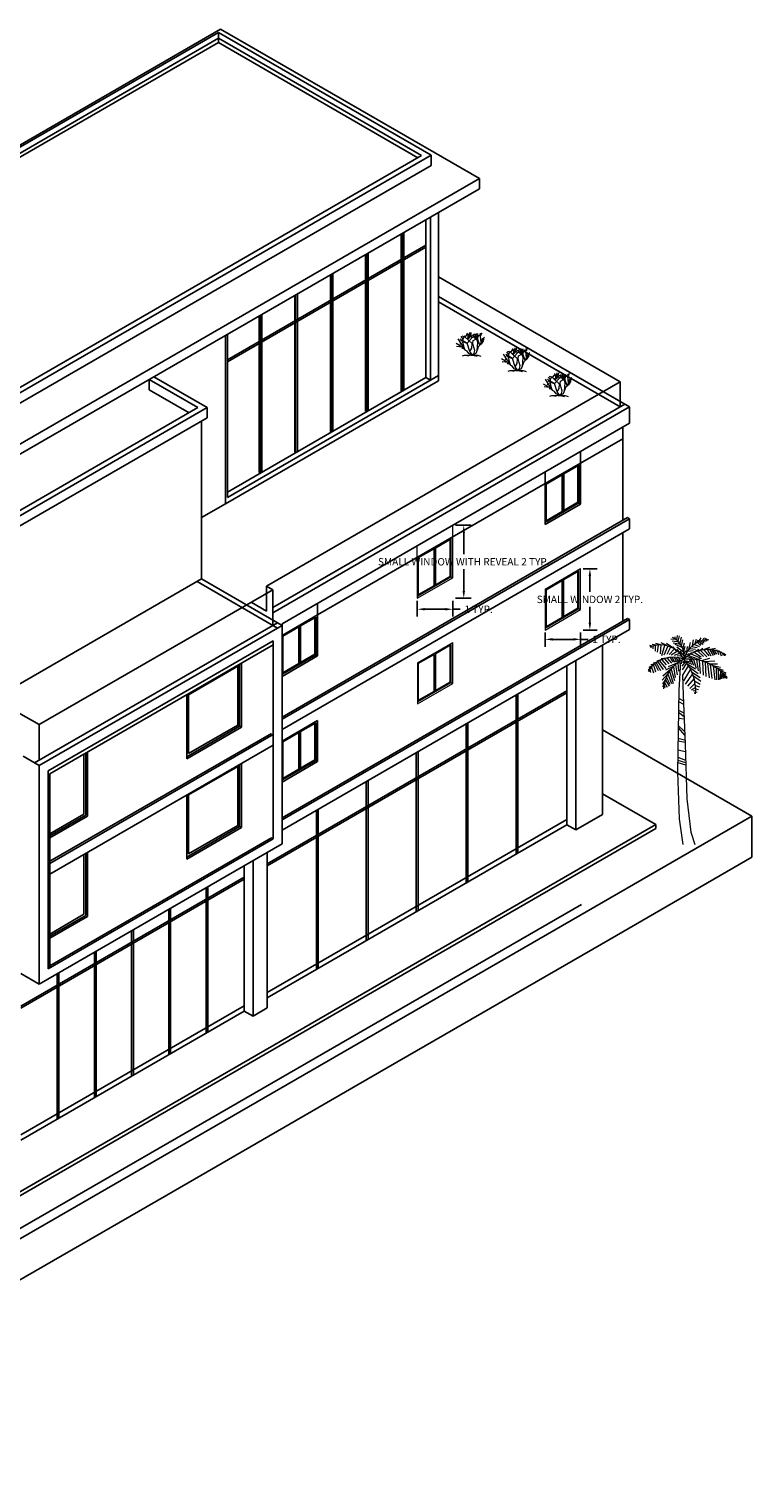
# Model space of a CAD drawing. Units: metres. Extents: x 20738 to 41533, y 14777 to 29586.
# Tile 2 of 2: x 20763 to 20780, y 14778 to 14814. Entities that reach past the tile are written whole.
import ezdxf

# ---------------------------------------------------------------- set-up
doc = ezdxf.new("R2010")
doc.units = ezdxf.units.M
for name, color, linetype, lineweight in [('A-ANNO-DIMS', 2, 'Continuous', 18), ('A-ANNO-NPLT', 8, 'Continuous', 13), ('A-ELEV', 7, 'Continuous', 25), ('A-GLAZ', 4, 'Continuous', 18), ('L-PLNT', 92, 'Continuous', 13)]:
    doc.layers.add(name, color=color, linetype=linetype, lineweight=lineweight)
doc.styles.get("Standard").update_dxf_attribs({"font": 'arial.ttf'})
doc.dimstyles.get("Standard").update_dxf_attribs({"dimtxt": 0.18, "dimasz": 0.18, "dimexe": 0.18, "dimexo": 0.0625, "dimgap": 0.09, "dimtad": 0, "dimtih": 1, "dimtoh": 1, "dimdec": 4, "dimzin": 0, "dimdsep": 46, "dimtxsty": 'Standard', "dimcen": 0.09, "dimadec": 0, "dimazin": 0, "dimtfac": 1, "dimtdec": 4, "dimtofl": 0, "dimtmove": 0, "dimatfit": 3, "dimfxl": 1, "dimtolj": 1, "dimtzin": 0, "dimarcsym": 0})

# ---------------------------------------------------------------- blocks, each defined once
blk = doc.blocks.new('*U2')
for p, q in [((-18.24, 11.04), (-21.755, 16.655)), ((-12.96, 12.48), (-19.68, 16.32)), ((-13.92, 12.48), (-19.2, 14.88)), ((-16.8, 16.32), (-18.72, 18.72)), ((-14.88, 18.24), (-17.76, 19.2)), ((-16.8, 16.32), (-15.36, 19.68)), ((-16.8, 12.48), (-16.8, 16.32)), ((-14.88, 18.24), (-12.96, 20.64)), ((-8.16, 12), (-14.88, 18.24)), ((-13.325, 16.724), (-11.433, 18.289)), ((-12.96, 12.48), (-8.16, 17.76)), ((-12.471, 19.775), (-12.898, 22.044)), ((-11.677, 19.071), (-12.471, 19.775)), ((-11.28, 19.619), (-12.104, 21.184)), ((-12.043, 15.628), (-11.921, 18.836)), ((-11.982, 16.802), (-10.579, 18.054)), ((-11.921, 18.836), (-10.64, 20.401)), ((-11.433, 18.289), (-10.457, 22.749)), ((-10.579, 18.054), (-9.846, 19.697)), ((-8.16, 17.76), (-10.56, 21.6)), ((-9.48, 19.775), (-8.992, 22.592)), ((-7.2, 19.68), (-8.64, 20.16)), ((-8.16, 17.76), (-5.28, 19.2)), ((-7.68, 12.48), (-7.2, 14.88)), ((-7.2, 19.68), (-6.24, 21.12)), ((-4.8, 16.32), (-7.2, 19.68)), ((-7.2, 14.88), (-3.84, 16.8)), ((-5.086, 17.741), (-5.513, 21.34)), ((-5.28, 19.2), (-3.84, 21.6)), ((-3.377, 15.315), (-5.086, 17.819)), ((-2.88, 12.96), (-4.32, 19.68)), ((-3.84, 16.8), (-0.96, 20.64)), ((-3.377, 18.602), (-2.888, 21.575)), ((-2.766, 16.802), (-3.377, 18.602)), ((-2.88, 15.84), (-2.4, 20.16)), ((-0.96, 10.56), (-2.88, 15.84)), ((-0.508, 21.888), (-0.081, 20.558)), ((-0.203, 19.149), (0.102, 21.34)), ((0.346, 13.203), (-0.203, 19.149)), ((-0.142, 19.384), (0.59, 20.401)), ((-0.02, 20.01), (0.896, 21.105)), ((0.041, 20.714), (1.384, 22.044)), ((0.102, 21.34), (0.835, 21.888)), ((0.346, 13.203), (1.323, 16.254)), ((0.96, 12), (1.44, 15.36)), ((0.96, 12), (2.88, 14.88)), ((1.323, 16.254), (3.642, 18.289)), ((1.44, 15.36), (2.88, 17.28)), ((1.92, 13.44), (2.4, 15.36)), ((2.4, 15.36), (3.36, 16.32)), ((-17.76, 8.64), (-23.663, 11.961)), ((-17.76, 8.64), (-23.128, 9.222)), ((-18.24, 11.04), (-20.16, 11.52)), ((-15.84, 8.16), (-18.24, 11.04)), ((-16.32, 7.2), (-18.24, 7.2)), ((-16.8, 12.48), (-17.76, 12.96)), ((-14.88, 5.76), (-17.76, 8.64)), ((-15.84, 0.48), (-17.76, 0)), ((-15.84, 8.16), (-16.8, 12.48)), ((-14.88, 5.76), (-15.84, 8.16)), ((-13.44, 0.48), (-15.84, 0.48)), ((-12.96, 4.8), (-14.88, 5.76)), ((-12.96, 12.48), (-13.92, 12.48)), ((-9.6, 0.96), (-13.44, 0.48)), ((-10.56, 4.32), (-12.96, 12.48)), ((-11.52, 2.4), (-12.96, 4.8)), ((-9.6, 0.96), (-12.96, 0)), ((-8.64, 0.96), (-11.52, 2.4)), ((-10.56, 4.32), (-8.64, 7.68)), ((-8.64, 1.92), (-10.56, 4.32)), ((-9.6, 0.96), (-7.68, 0.96)), ((-8.64, 7.68), (-8.16, 12)), ((-8.64, 0.96), (-4.32, 2.88)), ((-8.64, 0.96), (-6.24, 2.88)), ((-8.64, 0.96), (-8.64, 1.92)), ((-8.64, 0.96), (-2.88, 0.96)), ((-6.72, 8.64), (-7.68, 12.48)), ((-7.68, 0.96), (-6.24, 0.48)), ((-5.76, 5.28), (-6.72, 8.64)), ((-6.24, 2.88), (-5.76, 5.28)), ((-6.24, 0.48), (-3.36, 0)), ((-4.32, 2.88), (-1.92, 9.6)), ((-3.36, 5.28), (-2.88, 12.96)), ((-2.88, 0.96), (0, 0)), ((-1.92, 9.6), (0.96, 12)), ((-0.48, 10.8), (0.346, 13.203))]:
    blk.add_line(p, q)
blk = doc.blocks.new('*U4')
for p, q in [((-6.727, 197.202), (-11.366, 197.45)), ((-3.441, 194.477), (-10.013, 195.716)), ((-7.5, 199.68), (-7.5, 197.946)), ((-5.567, 196.707), (-4.987, 201.167)), ((-4.407, 195.716), (-3.247, 200.672)), ((-2.474, 193.733), (-1.315, 199.433)), ((-1.121, 190.759), (0.232, 196.955)), ((9.317, 191.255), (10.283, 196.955)), ((11.829, 192.99), (13.182, 197.45)), ((13.956, 194.229), (14.729, 196.955)), ((15.116, 194.477), (17.822, 198.689)), ((18.015, 195.716), (20.914, 198.689)), ((19.368, 196.459), (19.948, 193.733)), ((20.914, 196.459), (21.301, 194.972)), ((21.301, 196.459), (22.847, 198.441)), ((22.074, 196.707), (23.427, 195.716)), ((23.234, 196.707), (23.62, 197.698)), ((-29.729, 190.759), (-31.469, 191.255)), ((-30.309, 190.512), (-30.695, 189.025)), ((-25.283, 191.751), (-29.342, 192.246)), ((-28.763, 190.759), (-28.763, 188.281)), ((-26.443, 191.503), (-26.636, 186.051)), ((-20.064, 191.751), (-25.863, 193.238)), ((-23.737, 191.751), (-24.51, 185.06)), ((-21.031, 191.998), (-21.804, 183.325)), ((-15.232, 191.255), (-20.644, 193.981)), ((-17.551, 191.503), (-20.451, 181.343)), ((-14.265, 190.759), (-18.131, 182.086)), ((-9.433, 189.025), (-15.618, 193.238)), ((-11.753, 189.768), (-15.425, 182.83)), ((-8.08, 188.034), (-12.912, 182.83)), ((-4.987, 185.803), (-10.979, 182.086)), ((-1.894, 192.494), (-9.24, 193.733)), ((-6.147, 186.299), (-9.24, 190.264)), ((-3.247, 183.821), (-8.08, 181.838)), ((-0.541, 189.52), (-7.307, 192.494)), ((-5.76, 190.016), (0.618, 185.308)), ((-5.76, 188.034), (-1.508, 182.582)), ((-2.668, 185.803), (1.198, 181.343)), ((0.038, 188.281), (1.778, 193.981)), ((1.005, 185.803), (2.358, 190.759)), ((1.005, 182.582), (2.938, 186.547)), ((2.938, 182.582), (6.61, 183.821)), ((4.098, 185.06), (4.678, 190.512)), ((4.871, 186.051), (10.09, 186.547)), ((4.871, 181.591), (8.544, 184.812)), ((5.644, 181.838), (13.569, 178.865)), ((5.837, 187.786), (7.577, 194.229)), ((6.997, 188.529), (12.216, 187.786)), ((7.77, 183.325), (16.082, 179.856)), ((8.544, 190.512), (13.763, 189.52)), ((9.51, 184.317), (15.502, 188.034)), ((11.25, 192.494), (15.889, 190.512)), ((11.25, 184.812), (17.628, 180.352)), ((14.536, 193.981), (17.242, 191.255)), ((14.536, 185.803), (19.948, 180.847)), ((15.695, 186.299), (19.368, 188.777)), ((16.082, 194.972), (17.822, 192.494)), ((17.242, 186.547), (23.041, 180.599)), ((18.015, 195.468), (18.981, 192.494)), ((19.368, 187.29), (26.133, 189.768)), ((20.721, 187.042), (25.167, 181.343)), ((23.814, 187.29), (26.907, 181.343)), ((24.78, 187.538), (31.546, 188.777)), ((26.133, 187.29), (29.419, 181.838)), ((28.066, 187.29), (30.966, 182.582)), ((29.806, 186.795), (32.319, 183.078)), ((29.999, 186.795), (33.092, 187.29)), ((32.512, 186.299), (35.218, 186.299)), ((33.479, 186.051), (34.445, 182.83)), ((35.605, 185.556), (37.151, 185.308)), ((35.798, 185.308), (36.958, 181.591)), ((38.118, 184.317), (38.504, 181.838)), ((39.857, 182.83), (40.244, 181.591)), ((-32.628, 167.961), (-33.208, 167.961)), ((-32.628, 167.713), (-32.435, 165.979)), ((-28.956, 172.174), (-32.435, 170.192)), ((-31.082, 169.944), (-32.435, 169.2)), ((-31.662, 168.705), (-31.082, 165.483)), ((-27.409, 173.413), (-30.695, 172.67)), ((-29.922, 170.687), (-27.989, 165.235)), ((-25.09, 175.148), (-28.376, 174.404)), ((-27.989, 172.422), (-26.056, 166.227)), ((-26.829, 173.661), (-23.544, 167.218)), ((-25.476, 174.652), (-21.224, 167.466)), ((-21.031, 177.626), (-24.897, 176.387)), ((-24.317, 175.891), (-18.711, 168.457)), ((-22.191, 176.635), (-16.391, 169.448)), ((-15.618, 179.36), (-20.644, 178.617)), ((-20.064, 177.626), (-15.812, 172.67)), ((-12.139, 167.961), (-19.098, 162.014)), ((-17.358, 178.617), (-13.299, 173.661)), ((-8.466, 171.678), (-16.585, 167.713)), ((-15.038, 179.36), (-10.786, 174.404)), ((-4.214, 175.148), (-14.072, 170.935)), ((-12.332, 180.104), (-9.433, 175.643)), ((-10.979, 168.457), (-7.887, 157.801)), ((-10.206, 180.104), (-8.08, 175.891)), ((-8.853, 170.935), (-7.113, 160.527)), ((-1.701, 176.882), (-8.66, 175.396)), ((-8.273, 180.104), (-6.147, 176.635)), ((-6.92, 172.917), (-5.374, 163.253)), ((-6.34, 179.608), (-4.6, 177.13)), ((-1.315, 181.591), (-5.374, 181.095)), ((-4.6, 174.9), (-4.021, 166.722)), ((-4.021, 179.36), (-2.861, 177.378)), ((-2.668, 176.387), (-2.376, 170.594)), ((-0.348, 180.352), (-1.894, 180.104)), ((-0.928, 176.882), (-1.508, 173.909)), ((2.551, 175.891), (-0.928, 171.431)), ((3.711, 174.404), (-0.541, 167.961)), ((5.257, 171.926), (-0.155, 163.005)), ((1.585, 177.13), (0.038, 174.652)), ((7.384, 168.705), (0.812, 157.553)), ((1.585, 177.13), (6.61, 176.139)), ((2.938, 175.891), (8.737, 173.413)), ((4.098, 180.847), (8.35, 179.608)), ((4.291, 173.909), (12.216, 168.953)), ((6.224, 178.121), (8.157, 175.148)), ((6.417, 170.439), (14.729, 164.492)), ((7.384, 178.369), (10.476, 179.36)), ((8.157, 178.121), (10.476, 172.422)), ((10.476, 177.874), (12.796, 169.696)), ((11.829, 177.874), (18.015, 179.113)), ((13.182, 177.874), (14.729, 166.97)), ((15.889, 177.13), (16.855, 164.492)), ((18.015, 177.13), (26.133, 179.113)), ((18.981, 175.891), (19.561, 163.005)), ((20.914, 175.891), (30.966, 176.635)), ((21.688, 175.396), (22.074, 161.518)), ((23.814, 174.404), (25.554, 160.279)), ((25.554, 173.661), (33.285, 173.661)), ((26.52, 173.165), (28.066, 159.784)), ((28.839, 172.174), (36.378, 170.687)), ((29.226, 171.926), (30.966, 158.545)), ((30.966, 170.687), (38.891, 167.713)), ((32.126, 169.696), (32.512, 158.545)), ((34.058, 168.705), (34.445, 158.545)), ((35.412, 167.713), (41.404, 164.988)), ((-14.265, 164.244), (-19.678, 158.049)), ((-16.005, 160.031), (-19.484, 154.084)), ((-17.358, 155.819), (-14.845, 151.358)), ((-16.585, 158.545), (-13.106, 152.35)), ((-15.618, 160.775), (-12.332, 154.332)), ((-14.265, 163.749), (-10.786, 154.828)), ((-12.719, 166.722), (-9.046, 154.828)), ((9.317, 164.244), (2.358, 154.332)), ((10.863, 159.784), (4.484, 152.35)), ((11.829, 155.075), (6.804, 150.119)), ((8.544, 165.979), (16.662, 160.527)), ((10.09, 162.51), (17.435, 157.058)), ((11.443, 157.553), (16.855, 154.332)), ((36.378, 166.474), (35.605, 158.792)), ((37.731, 165.235), (36.958, 159.288)), ((37.924, 165.235), (41.404, 163.749)), ((38.504, 164.492), (38.504, 159.536)), ((39.664, 163.253), (42.37, 161.766)), ((39.857, 162.757), (39.857, 160.031)), ((40.824, 161.766), (41.21, 160.031)), ((41.21, 161.518), (42.757, 160.279)), ((-18.131, 153.589), (-19.484, 151.606)), ((-17.938, 152.597), (-16.972, 151.111)), ((-4.081, 140.645), (0.753, 138.261)), ((12.603, 151.111), (8.544, 148.385)), ((12.216, 148.137), (10.09, 147.393)), ((12.409, 145.659), (11.056, 145.659)), ((12.216, 153.093), (16.082, 151.606)), ((12.409, 146.898), (13.763, 146.402)), ((12.603, 149.872), (15.116, 149.128)), ((-4.081, 137.547), (0.753, 135.163)), ((-4.081, 129.205), (1.124, 126.821)), ((-4.081, 127.298), (1.31, 123.246)), ((-4.453, 112.283), (1.682, 105.133)), ((-4.267, 114.428), (1.682, 108.708)), ((-4.081, 121.578), (1.31, 120.863)), ((-4.639, 102.273), (1.868, 100.604)), ((-4.453, 99.651), (2.24, 98.459)), ((-4.825, 83.921), (2.612, 81.061)), ((-4.453, 91.071), (2.426, 89.641)), ((-4.639, 81.299), (2.797, 78.916)), ((-4.639, 78.916), (2.797, 76.771))]:
    blk.add_line(p, q)
for points in [[(-2.363, 170.553), (-3.88, 148.505), (-4.988, 69.634), (-3.325, 24.869), (0, 0)], [(-0.116, 162.848), (0.554, 143.532), (2.217, 96.635), (3.88, 44.054), (7.76, 12.079), (11.64, 0)]]:
    blk.add_lwpolyline(points)
for centre, radius, start, end in [((-18.427, 181.448), 19.715, 350.285, 64.11229), ((25.595, 171.567), 25.395, 91.40319, 163.882), ((-21.738, 166.094), 25.899, 27.67115, 112.5305), ((23.687, 155.341), 32.188, 56.19272, 134.3213), ((-9.259, 151.732), 28.386, 68.38311, 147.5322), ((14.394, 148.393), 32.752, 113.7592, 177.4133), ((5.828, 132.718), 45.639, 35.98777, 95.82273), ((-32.8, 147.923), 45.309, 356.1943, 41.37848)]:
    blk.add_arc(centre, radius, start, end)
blk = doc.blocks.new('WIN-SMALL')
for p, q in [((0, 1), (0.866, 1.5)), ((0.454, 1.235), (0.822, 1.448)), ((0.8, 0.54), (0.8, 1.435)), ((0.822, 0.525), (0.822, 1.448)), ((0.866, 0.5), (0.866, 1.5)), ((0.021, 0.985), (0.411, 1.21)), ((0.411, 0.315), (0.411, 1.21)), ((0.454, 0.34), (0.454, 1.235)), ((0, 1), (0, 0)), ((0.021, 0.985), (0.021, 0.062)), ((0, 0), (0.866, 0.5)), ((0.021, 0.062), (0.822, 0.525)), ((0.454, 0.34), (0.8, 0.54)), ((0.798, 0.538), (0.866, 0.5)), ((0.021, 0.09), (0.411, 0.315))]:
    blk.add_line(p, q)
blk = doc.blocks.new('WIN-SMALL-REVEAL')
for p, q in [((0.866, 1.5), (0.866, 1.784)), ((0, 1), (0.866, 1.5)), ((0.455, 1.235), (0.823, 1.448)), ((0.801, 0.54), (0.801, 1.435)), ((0.823, 0.525), (0.823, 1.448)), ((0.866, 0.5), (0.866, 1.5)), ((0, 1), (0, 1.284)), ((0.022, 0.985), (0.412, 1.21)), ((0.412, 0.315), (0.412, 1.21)), ((0.455, 0.34), (0.455, 1.235)), ((0, 1), (0, 0)), ((0.022, 0.985), (0.022, 0.062)), ((0, 0), (0.866, 0.5)), ((0.022, 0.062), (0.823, 0.525)), ((0.455, 0.34), (0.801, 0.54)), ((0.799, 0.539), (0.866, 0.5)), ((0.022, 0.09), (0.412, 0.315))]:
    blk.add_line(p, q)
blk = doc.blocks.new('*D7')
at = {"layer": 'A-ANNO-DIMS', "color": 0, "lineweight": -2, "transparency": 16777216}
for p, q in [((20776.049, 14800.805), (20776.392, 14800.805)), ((20776.212, 14800.625), (20776.212, 14800.238)), ((20776.212, 14799.485), (20776.212, 14799.872)), ((20776.049, 14799.305), (20776.392, 14799.305))]:
    blk.add_line(p, q, dxfattribs=at)
at = {"layer": 'A-ANNO-DIMS', "color": 0, "transparency": 16777216}
for points in [[(20776.182, 14800.625), (20776.242, 14800.625), (20776.212, 14800.805)], [(20776.182, 14799.485), (20776.242, 14799.485), (20776.212, 14799.305)]]:
    blk.add_solid(points, dxfattribs=at)
at = {"layer": 'Defpoints', "color": 0, "transparency": 16777216}
for p in [(20775.987, 14800.805), (20776.212, 14800.805), (20775.987, 14799.305)]:
    blk.add_point(p, dxfattribs=at)
at = {"layer": 'A-ANNO-DIMS', "color": 0, "transparency": 16777216, "insert": (20776.212, 14800.055), "char_height": 0.18, "attachment_point": 5}
blk.add_mtext('\\A1;SMALL WINDOW 2 TYP.', dxfattribs=at)
blk = doc.blocks.new('*D8')
at = {"layer": 'A-ANNO-DIMS', "color": 0, "lineweight": -2, "transparency": 16777216}
for p, q in [((20775.121, 14799.243), (20775.121, 14798.9)), ((20775.987, 14799.243), (20775.987, 14798.9)), ((20775.301, 14799.08), (20775.807, 14799.08)), ((20775.987, 14799.08), (20776.167, 14799.08))]:
    blk.add_line(p, q, dxfattribs=at)
at = {"layer": 'A-ANNO-DIMS', "color": 0, "transparency": 16777216}
for points in [[(20775.301, 14799.11), (20775.301, 14799.05), (20775.121, 14799.08)], [(20775.807, 14799.11), (20775.807, 14799.05), (20775.987, 14799.08)]]:
    blk.add_solid(points, dxfattribs=at)
at = {"layer": 'Defpoints', "color": 0, "transparency": 16777216}
for p in [(20775.121, 14799.305), (20775.987, 14799.305), (20775.987, 14799.08)]:
    blk.add_point(p, dxfattribs=at)
at = {"layer": 'A-ANNO-DIMS', "color": 0, "transparency": 16777216, "insert": (20776.616, 14799.08), "char_height": 0.18, "attachment_point": 5}
blk.add_mtext('\\A1;1 TYP.', dxfattribs=at)
blk = doc.blocks.new('*D9')
at = {"layer": 'A-ANNO-DIMS', "color": 0, "lineweight": -2, "transparency": 16777216}
for p, q in [((20772.928, 14801.867), (20773.313, 14801.867)), ((20773.133, 14801.687), (20773.133, 14801.158)), ((20773.133, 14800.262), (20773.133, 14800.791)), ((20772.928, 14800.082), (20773.313, 14800.082))]:
    blk.add_line(p, q, dxfattribs=at)
at = {"layer": 'A-ANNO-DIMS', "color": 0, "transparency": 16777216}
for points in [[(20773.103, 14801.687), (20773.163, 14801.687), (20773.133, 14801.867)], [(20773.103, 14800.262), (20773.163, 14800.262), (20773.133, 14800.082)]]:
    blk.add_solid(points, dxfattribs=at)
at = {"layer": 'Defpoints', "color": 0, "transparency": 16777216}
for p in [(20772.865, 14801.867), (20773.133, 14801.867), (20772.865, 14800.082)]:
    blk.add_point(p, dxfattribs=at)
at = {"layer": 'A-ANNO-DIMS', "color": 0, "transparency": 16777216, "insert": (20773.133, 14800.974), "char_height": 0.18, "attachment_point": 5}
blk.add_mtext('\\A1;SMALL WINDOW WITH REVEAL 2 TYP.', dxfattribs=at)
blk = doc.blocks.new('*D10')
at = {"layer": 'A-ANNO-DIMS', "color": 0, "lineweight": -2, "transparency": 16777216}
for p, q in [((20771.999, 14800.02), (20771.999, 14799.635)), ((20772.865, 14800.02), (20772.865, 14799.635)), ((20772.179, 14799.815), (20772.685, 14799.815)), ((20772.865, 14799.815), (20773.045, 14799.815))]:
    blk.add_line(p, q, dxfattribs=at)
at = {"layer": 'A-ANNO-DIMS', "color": 0, "transparency": 16777216}
for points in [[(20772.179, 14799.845), (20772.179, 14799.785), (20771.999, 14799.815)], [(20772.685, 14799.845), (20772.685, 14799.785), (20772.865, 14799.815)]]:
    blk.add_solid(points, dxfattribs=at)
at = {"layer": 'Defpoints', "color": 0, "transparency": 16777216}
for p in [(20771.999, 14800.082), (20772.865, 14800.082), (20772.865, 14799.815)]:
    blk.add_point(p, dxfattribs=at)
at = {"layer": 'A-ANNO-DIMS', "color": 0, "transparency": 16777216, "insert": (20773.495, 14799.815), "char_height": 0.18, "attachment_point": 5}
blk.add_mtext('\\A1;1 TYP.', dxfattribs=at)

msp = doc.modelspace()

# ---------------------------------------------------------------- linework, layer by layer
at = {"layer": 'A-ANNO-NPLT'}
for p in [(20774.434, 14793.851), (20773.214, 14793.147), (20771.994, 14792.442), (20770.775, 14791.738), (20769.555, 14791.034), (20766.863, 14789.48), (20765.954, 14788.955), (20765.044, 14788.43), (20764.135, 14787.905), (20763.225, 14787.38)]:
    msp.add_point(p, dxfattribs=at)
at = {"layer": 'A-ELEV'}
for p, q in [((20767.197, 14813.979), (20745.234, 14801.298)), ((20761.514, 14810.649), (20767.143, 14813.899)), ((20767.143, 14813.899), (20772.339, 14810.899)), ((20767.143, 14813.649), (20767.143, 14813.899)), ((20767.197, 14813.979), (20773.518, 14810.329)), ((20746.597, 14801.891), (20767.143, 14813.754)), ((20761.514, 14810.399), (20767.143, 14813.649)), ((20767.143, 14813.754), (20772.101, 14810.891)), ((20767.143, 14813.649), (20772.01, 14810.839)), ((20772.339, 14810.899), (20751.555, 14798.899)), ((20772.101, 14810.891), (20751.555, 14799.029)), ((20772.339, 14810.649), (20751.555, 14798.649)), ((20772.339, 14810.899), (20772.339, 14810.649)), ((20751.555, 14797.649), (20773.518, 14810.329)), ((20773.518, 14810.329), (20773.518, 14810.079)), ((20751.555, 14797.399), (20773.518, 14810.079)), ((20772.209, 14809.324), (20772.209, 14805.476)), ((20772.322, 14809.389), (20772.322, 14805.411)), ((20772.513, 14809.499), (20772.513, 14805.391)), ((20771.603, 14805.151), (20771.603, 14808.974)), ((20771.625, 14805.138), (20771.625, 14808.986)), ((20771.668, 14805.163), (20771.668, 14809.011)), ((20772.209, 14808.703), (20767.362, 14805.904)), ((20772.209, 14808.653), (20767.362, 14805.854)), ((20770.734, 14804.649), (20770.734, 14808.472)), ((20770.756, 14804.636), (20770.756, 14808.484)), ((20770.802, 14804.663), (20770.802, 14808.511)), ((20769.876, 14804.153), (20769.876, 14807.977)), ((20769.898, 14804.141), (20769.898, 14807.989)), ((20769.936, 14804.163), (20769.936, 14808.011)), ((20776.951, 14805.365), (20772.513, 14807.928)), ((20769.005, 14803.651), (20769.005, 14807.474)), ((20769.027, 14803.638), (20769.027, 14807.486)), ((20769.07, 14803.663), (20769.07, 14807.511)), ((20772.513, 14807.448), (20777.176, 14804.755)), ((20772.513, 14807.318), (20776.951, 14804.755)), ((20768.139, 14803.151), (20768.139, 14806.974)), ((20768.161, 14803.138), (20768.161, 14806.986)), ((20768.204, 14803.163), (20768.204, 14807.011)), ((20767.316, 14802.391), (20767.316, 14806.499)), ((20767.362, 14802.547), (20767.362, 14806.52)), ((20765.455, 14805.424), (20766.641, 14804.739)), ((20765.455, 14805.424), (20765.455, 14805.174)), ((20765.568, 14805.489), (20766.867, 14804.739)), ((20772.513, 14805.391), (20767.316, 14802.391)), ((20772.513, 14805.521), (20767.362, 14802.547)), ((20772.209, 14805.476), (20767.362, 14802.677)), ((20768.316, 14800.38), (20776.951, 14805.365)), ((20772.322, 14805.411), (20772.209, 14805.476)), ((20776.951, 14804.755), (20776.951, 14805.365)), ((20765.455, 14805.174), (20766.425, 14804.614)), ((20771.625, 14805.138), (20771.603, 14805.151)), ((20760.804, 14801.239), (20766.867, 14804.739)), ((20760.804, 14801.369), (20766.641, 14804.739)), ((20766.867, 14804.739), (20766.867, 14804.489)), ((20768.47, 14799.859), (20777.063, 14804.82)), ((20768.47, 14799.729), (20777.176, 14804.755)), ((20770.756, 14804.636), (20770.734, 14804.649)), ((20777.176, 14804.755), (20777.176, 14804.355)), ((20760.804, 14800.989), (20766.867, 14804.489)), ((20766.733, 14804.412), (20766.733, 14800.554)), ((20768.696, 14799.459), (20777.176, 14804.355)), ((20777.017, 14804.264), (20777.017, 14801.985)), ((20769.898, 14804.141), (20769.876, 14804.153)), ((20775.987, 14803.384), (20777.017, 14803.979)), ((20769.027, 14803.638), (20769.005, 14803.651)), ((20775.987, 14803.384), (20775.987, 14803.669)), ((20768.161, 14803.138), (20768.139, 14803.151)), ((20775.121, 14802.884), (20775.987, 14803.384)), ((20775.121, 14802.884), (20775.121, 14803.169)), ((20775.554, 14802.184), (20775.554, 14803.134)), ((20775.575, 14803.12), (20775.943, 14803.332)), ((20775.922, 14802.425), (20775.922, 14803.32)), ((20775.943, 14802.409), (20775.943, 14803.332)), ((20775.987, 14802.384), (20775.987, 14803.384)), ((20769.562, 14799.675), (20775.121, 14802.884)), ((20775.121, 14802.884), (20775.121, 14801.884)), ((20775.142, 14802.87), (20775.532, 14803.095)), ((20775.142, 14802.87), (20775.142, 14801.947)), ((20775.532, 14802.2), (20775.532, 14803.095)), ((20775.575, 14802.225), (20775.575, 14803.12)), ((20775.575, 14802.225), (20775.922, 14802.425)), ((20775.919, 14802.423), (20775.987, 14802.384)), ((20767.316, 14802.391), (20766.733, 14802.054)), ((20775.121, 14801.884), (20775.987, 14802.384)), ((20775.142, 14801.947), (20775.943, 14802.409)), ((20775.142, 14801.975), (20775.532, 14802.2)), ((20777.133, 14802.051), (20768.696, 14797.18)), ((20777.176, 14802.026), (20768.696, 14797.13)), ((20777.176, 14801.776), (20768.696, 14796.88)), ((20777.133, 14802.051), (20777.176, 14802.026)), ((20777.176, 14801.776), (20777.176, 14802.026)), ((20777.017, 14801.685), (20777.017, 14799.525)), ((20772.432, 14800.382), (20772.432, 14801.332)), ((20760.804, 14797.131), (20766.733, 14800.554)), ((20766.621, 14800.489), (20768.583, 14799.356)), ((20766.733, 14800.554), (20768.696, 14799.421)), ((20768.316, 14800.38), (20768.47, 14800.291)), ((20768.316, 14799.77), (20768.316, 14800.38)), ((20775.554, 14799.605), (20775.554, 14800.555)), ((20762.767, 14796.998), (20768.47, 14800.291)), ((20767.942, 14799.986), (20768.316, 14799.77)), ((20768.47, 14799.421), (20768.47, 14800.291)), ((20769.562, 14799.675), (20769.562, 14799.959)), ((20768.696, 14799.175), (20769.562, 14799.675)), ((20768.696, 14794.721), (20777.133, 14799.592)), ((20769.15, 14799.41), (20769.518, 14799.623)), ((20769.496, 14798.715), (20769.496, 14799.61)), ((20769.518, 14798.7), (20769.518, 14799.623)), ((20769.562, 14798.675), (20769.562, 14799.675)), ((20777.176, 14799.567), (20777.133, 14799.592)), ((20762.654, 14796.063), (20768.583, 14799.486)), ((20762.767, 14795.998), (20768.696, 14799.421)), ((20768.696, 14794.671), (20777.176, 14799.567)), ((20768.696, 14799.175), (20768.696, 14799.459)), ((20768.696, 14799.421), (20768.696, 14794.086)), ((20768.696, 14794.421), (20777.176, 14799.317)), ((20768.717, 14799.16), (20769.107, 14799.385)), ((20769.107, 14798.49), (20769.107, 14799.385)), ((20769.129, 14798.475), (20769.129, 14799.425)), ((20769.15, 14798.515), (20769.15, 14799.41)), ((20777.176, 14799.567), (20777.176, 14799.317)), ((20762.983, 14795.873), (20768.479, 14799.046)), ((20763.026, 14795.798), (20768.479, 14798.946)), ((20768.479, 14799.046), (20768.479, 14794.211)), ((20768.696, 14799.175), (20768.696, 14798.175)), ((20768.717, 14799.16), (20768.717, 14798.237)), ((20776.519, 14798.938), (20776.519, 14794.805)), ((20768.696, 14798.175), (20769.562, 14798.675)), ((20768.717, 14798.237), (20769.518, 14798.7)), ((20769.15, 14798.515), (20769.496, 14798.715)), ((20769.494, 14798.714), (20769.562, 14798.675)), ((20772.432, 14797.803), (20772.432, 14798.753)), ((20775.87, 14798.563), (20775.87, 14794.43)), ((20766.413, 14797.728), (20767.618, 14798.424)), ((20767.618, 14798.449), (20767.618, 14796.985)), ((20767.661, 14798.474), (20767.661, 14796.96)), ((20767.705, 14798.499), (20767.705, 14796.935)), ((20768.717, 14798.265), (20769.107, 14798.49)), ((20775.653, 14798.438), (20775.653, 14794.555)), ((20768.336, 14793.599), (20775.653, 14797.823)), ((20766.369, 14797.728), (20766.369, 14796.164)), ((20766.413, 14797.753), (20766.413, 14796.289)), ((20768.336, 14793.549), (20775.653, 14797.773)), ((20774.412, 14793.838), (20774.412, 14797.721)), ((20774.455, 14793.863), (20774.455, 14797.746)), ((20762.263, 14797.289), (20762.767, 14796.998)), ((20762.767, 14796.128), (20762.767, 14796.998)), ((20768.436, 14796.784), (20763.026, 14793.661)), ((20768.479, 14796.759), (20763.026, 14793.611)), ((20767.661, 14796.96), (20766.369, 14796.214)), ((20767.705, 14796.935), (20766.369, 14796.164)), ((20766.413, 14796.289), (20767.618, 14796.985)), ((20767.705, 14796.935), (20767.618, 14796.985)), ((20768.696, 14796.596), (20769.562, 14797.096)), ((20768.696, 14796.596), (20768.696, 14796.88)), ((20768.717, 14796.581), (20769.107, 14796.806)), ((20769.107, 14795.911), (20769.107, 14796.806)), ((20769.129, 14795.896), (20769.129, 14796.846)), ((20769.15, 14796.831), (20769.518, 14797.044)), ((20769.15, 14795.936), (20769.15, 14796.831)), ((20769.496, 14796.136), (20769.496, 14797.031)), ((20769.518, 14796.121), (20769.518, 14797.044)), ((20769.562, 14796.096), (20769.562, 14797.096)), ((20773.192, 14793.134), (20773.192, 14797.017)), ((20773.236, 14793.159), (20773.236, 14797.042)), ((20776.519, 14796.871), (20780.169, 14794.764)), ((20768.479, 14796.499), (20763.026, 14793.351)), ((20768.696, 14796.596), (20768.696, 14795.596)), ((20768.717, 14796.581), (20768.717, 14795.658)), ((20762.376, 14796.224), (20762.767, 14795.998)), ((20763.859, 14796.279), (20763.859, 14794.814)), ((20763.902, 14796.304), (20763.902, 14794.789)), ((20763.946, 14796.329), (20763.946, 14794.764)), ((20767.705, 14796.052), (20767.705, 14794.487)), ((20768.696, 14795.596), (20769.562, 14796.096)), ((20768.717, 14795.658), (20769.518, 14796.121)), ((20769.15, 14795.936), (20769.496, 14796.136)), ((20769.494, 14796.135), (20769.562, 14796.096)), ((20771.973, 14792.43), (20771.973, 14796.313)), ((20772.016, 14792.455), (20772.016, 14796.338)), ((20762.767, 14795.998), (20762.767, 14790.663)), ((20762.983, 14795.873), (20762.983, 14791.038)), ((20763.026, 14795.798), (20763.026, 14791.063)), ((20766.413, 14795.281), (20767.618, 14795.977)), ((20767.618, 14796.002), (20767.618, 14794.537)), ((20767.661, 14796.027), (20767.661, 14794.512)), ((20768.717, 14795.686), (20769.107, 14795.911)), ((20770.753, 14791.726), (20770.753, 14795.609)), ((20770.797, 14791.751), (20770.797, 14795.634)), ((20766.369, 14795.281), (20766.369, 14793.716)), ((20766.413, 14795.306), (20766.413, 14793.841)), ((20776.519, 14795.312), (20777.825, 14794.559)), ((20751.972, 14778.485), (20780.169, 14794.764)), ((20763.859, 14794.814), (20763.026, 14794.334)), ((20763.902, 14794.789), (20763.026, 14794.284)), ((20763.946, 14794.764), (20763.026, 14794.234)), ((20768.336, 14790.46), (20775.653, 14794.685)), ((20769.534, 14791.022), (20769.534, 14794.905)), ((20769.577, 14791.047), (20769.577, 14794.93)), ((20776.519, 14794.805), (20775.87, 14794.43)), ((20779.952, 14794.889), (20780.169, 14794.764)), ((20780.169, 14793.764), (20780.169, 14794.764)), ((20753.939, 14780.768), (20777.825, 14794.559)), ((20753.939, 14780.673), (20777.825, 14794.463)), ((20767.661, 14794.512), (20766.369, 14793.766)), ((20767.705, 14794.487), (20766.369, 14793.716)), ((20766.413, 14793.841), (20767.618, 14794.537)), ((20767.705, 14794.487), (20767.618, 14794.537)), ((20768.336, 14790.33), (20775.653, 14794.555)), ((20775.87, 14794.43), (20775.653, 14794.555)), ((20777.825, 14794.559), (20777.825, 14794.463)), ((20762.767, 14790.663), (20768.696, 14794.086)), ((20762.983, 14791.038), (20768.479, 14794.211)), ((20763.026, 14791.113), (20768.436, 14794.236)), ((20768.479, 14794.211), (20768.436, 14794.236)), ((20763.859, 14793.831), (20763.859, 14792.367)), ((20763.902, 14793.856), (20763.902, 14792.342)), ((20763.946, 14793.881), (20763.946, 14792.317)), ((20767.773, 14793.554), (20767.773, 14790.005)), ((20767.989, 14793.679), (20767.989, 14789.88)), ((20768.336, 14793.879), (20768.336, 14790.08)), ((20776.705, 14791.764), (20780.169, 14793.764)), ((20767.773, 14793.274), (20762.316, 14790.123)), ((20767.773, 14793.224), (20762.316, 14790.073)), ((20766.842, 14789.468), (20766.842, 14793.016)), ((20766.885, 14789.493), (20766.885, 14793.041)), ((20751.756, 14778.61), (20776.005, 14792.61)), ((20765.932, 14788.942), (20765.932, 14792.491)), ((20765.976, 14788.967), (20765.976, 14792.516)), ((20763.859, 14792.367), (20763.026, 14791.886)), ((20763.902, 14792.342), (20763.026, 14791.836)), ((20763.946, 14792.317), (20763.026, 14791.786)), ((20765.023, 14788.417), (20765.023, 14791.966)), ((20765.066, 14788.442), (20765.066, 14791.991)), ((20764.113, 14787.892), (20764.113, 14791.441)), ((20764.157, 14787.917), (20764.157, 14791.466)), ((20771.075, 14788.514), (20776.705, 14791.764)), ((20762.316, 14790.923), (20762.767, 14790.663)), ((20763.204, 14787.367), (20763.204, 14790.916)), ((20763.247, 14787.392), (20763.247, 14790.941)), ((20767.773, 14790.135), (20762.316, 14786.985)), ((20767.773, 14790.005), (20762.316, 14786.855)), ((20767.989, 14789.88), (20767.773, 14790.005)), ((20767.989, 14789.88), (20768.336, 14790.08)), ((20765.879, 14785.514), (20771.075, 14788.514)), ((20761.116, 14782.764), (20765.879, 14785.514))]:
    msp.add_line(p, q, dxfattribs=at)

# ---------------------------------------------------------------- block references
at = {"layer": 'A-GLAZ'}
for name, p in [('WIN-SMALL-REVEAL', (20771.999, 14800.082)), ('WIN-SMALL', (20775.121, 14799.306)), ('WIN-SMALL', (20772, 14797.503))]:
    msp.add_blockref(name, p, dxfattribs=at)
at = {"layer": 'L-PLNT', "xscale": 0.0254, "yscale": 0.0254, "zscale": 0.0254}
for name, p in [('*U2', (20773.546, 14805.995)), ('*U2', (20774.656, 14805.622)), ('*U2', (20775.681, 14805.009)), ('*U4', (20778.479, 14794.068))]:
    msp.add_blockref(name, p, dxfattribs=at)

# ---------------------------------------------------------------- dimensions: what is measured, and where the dimension line sits
at = {"layer": 'A-ANNO-DIMS'}
for base, p1, p2, text, picture, middle in [((20773.133, 14801.867), (20772.865, 14800.082), (20772.865, 14801.867), 'SMALL WINDOW WITH REVEAL <> TYP.', '*D9', (20773.133, 14800.974)), ((20776.211771887, 14800.805145435), (20775.986771887, 14799.305145435), (20775.986771887, 14800.805145435), 'SMALL WINDOW <> TYP.', '*D7', (20776.211771887, 14800.055145435))]:
    dim = msp.add_linear_dim(base=base, p1=p1, p2=p2, angle=90, text=text, dimstyle='Standard', override={"dimdec": 0, "dimlfac": 1, "dimrnd": 0, "dimzin": 0, "dimdsep": 46, "dimlunit": 2}, dxfattribs=at)
    dim.commit()
    dim.dimension.update_dxf_attribs({"geometry": picture, "text_midpoint": middle})
for base, p1, p2, picture, middle in [((20772.865, 14799.815), (20771.999, 14800.082), (20772.865, 14800.082), '*D10', (20773.495, 14799.815)), ((20775.987, 14799.08), (20775.121, 14799.305), (20775.987, 14799.305), '*D8', (20776.616, 14799.08))]:
    dim = msp.add_linear_dim(base=base, p1=p1, p2=p2, text='<> TYP.', dimstyle='Standard', override={"dimdec": 0, "dimlfac": 1, "dimrnd": 0, "dimzin": 0, "dimdsep": 46, "dimlunit": 2}, dxfattribs=at)
    dim.commit()
    dim.dimension.update_dxf_attribs({"geometry": picture, "text_midpoint": middle})

doc.saveas('drawing.dxf')
